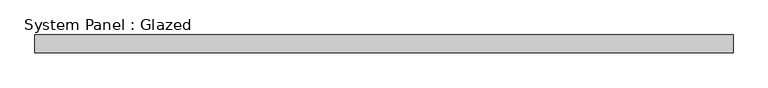
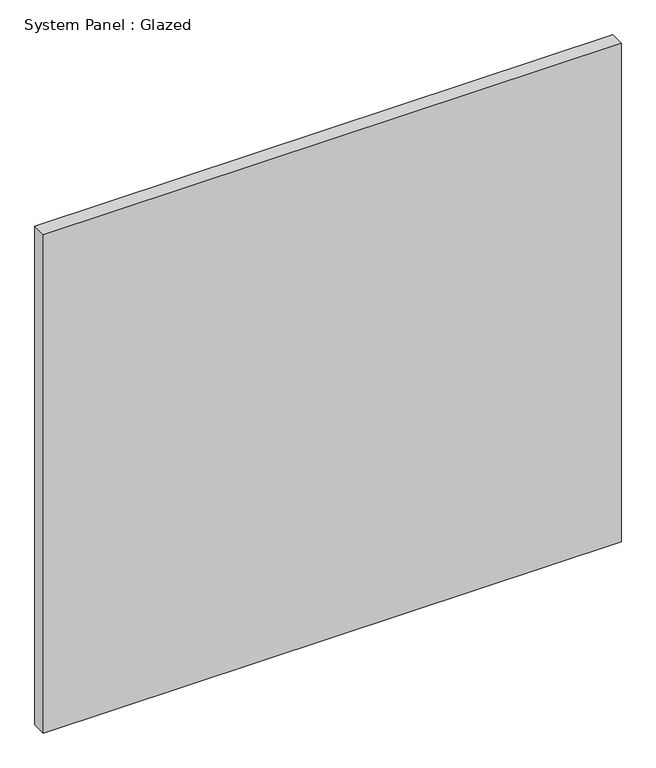
"""IFC4 building model written with IfcOpenShell, lengths in millimetres: plate geometry, System Panel : Glazed."""

from ifc_helpers import new_model, si_unit, origin, origin_with_axes, place, context, project, spatial, polyline, outline, extrude, source, transform, mapped, element, save


def system_panel_glazed_97d0a6f3(model_context):
    return source(origin(), model_context, "Body", "SweptSolid", [
        extrude(outline(polyline([(501.7180043, 19.05), (-501.7180043, 19.05), (-501.7180043, 44.45), (501.7180043, 44.45), (501.7180043, 19.05)])), origin_with_axes(), (0.0, 0.0, 1.0), 914.4),
    ])


if __name__ == "__main__":
    model = new_model("IFC4")
    model_context = context("Model", 3, world=origin())
    ifc_project = project(units=[si_unit("LENGTHUNIT", "METRE", prefix="MILLI")], contexts=[model_context])
    site = spatial("IfcSite", under=ifc_project)
    building = spatial("IfcBuilding", under=site)
    placement = place(None, origin())
    system_panel_glazed_shape = system_panel_glazed_97d0a6f3(model_context)
    element("IfcPlate", 1, ObjectType="System Panel : Glazed", at=placement, inside=building, context=model_context, shape_type="MappedRepresentation", body=[
        mapped(system_panel_glazed_shape, transform((0.0, 0.0, 0.0), x_axis=(1.0, 0.0, 0.0), y_axis=(0.0, 1.0, 0.0), z_axis=(0.0, 0.0, 1.0))),
    ])
    save(model, "model.ifc")

# Revit data of these elements
# Type "System Panel : Glazed"
#   Construction Type Id = "GSP4R"
#   Analytic Construction = "1/8 in Pilkington single glazing"
#   Visual Light Transmittance = 0.9
#   Solar Heat Gain Coefficient = 0.86
#   Heat Transfer Coefficient (U) = 1.18115 BTU/(h·ft²·°F)
# Element 1 (IfcPlate, "System Panel : Glazed")
#   Materials on its faces: "Glass"
# Materials
#   "Glass": class "Glass", colour RGB 0 128 192, transparency 0.75, Description = "Soda Lime Glass", Cost = 0
